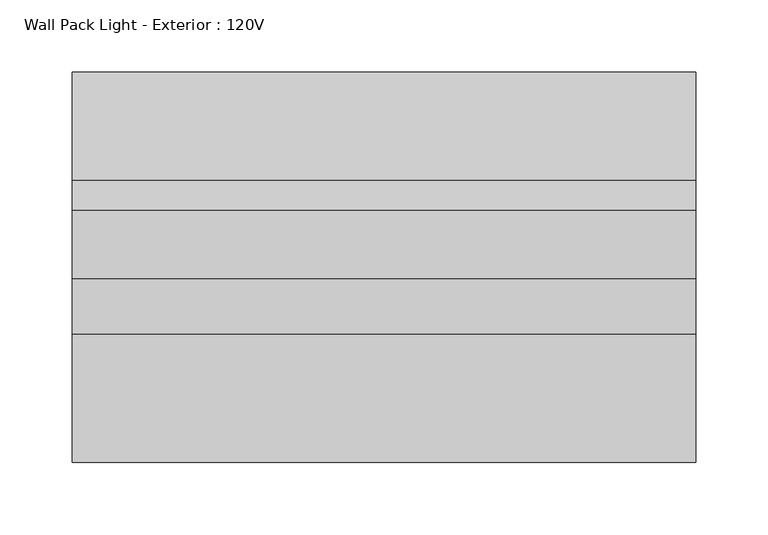
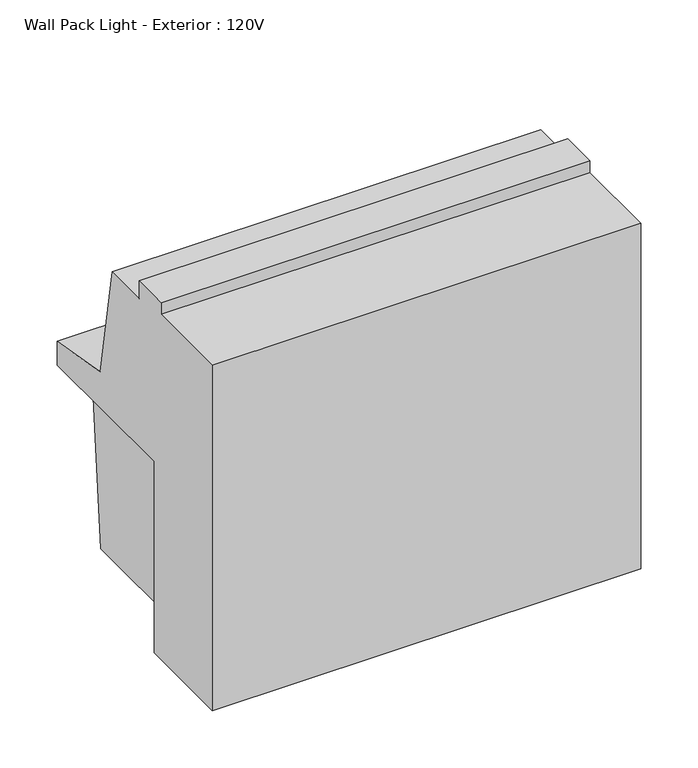
"""IFC4 building model written with IfcOpenShell, lengths in millimetres: light fixture geometry, Wall Pack Light - Exterior : 120V."""

from ifc_helpers import new_model, si_unit, frame, origin, place, context, project, spatial, polyline, outline, extrude, source, transform, mapped, element, save


def wall_pack_light_exterior_120v_50d39a1a(model_context):
    return source(origin(), model_context, "Body", "SweptSolid", [
        extrude(outline(polyline([(340.420745, 2393.95), (203.2, 2393.95), (203.2, 2578.1), (355.5170754, 2578.1), (340.420745, 2393.95)])), frame((-68.7349223, 0.0, 0.0), z_axis=(1.0, 0.0, 0.0), x_axis=(0.0, 1.0, 0.0)), (0.0, 0.0, 1.0), 380.9989788),
        extrude(outline(polyline([(190.5, 2755.9), (228.6, 2755.9), (228.6, 2736.85), (276.040971, 2736.85), (297.0426549, 2617.7435323), (372.0850056, 2604.5115412), (372.0850056, 2579.1115412), (203.2, 2579.1115412), (203.2, 2374.9), (101.6, 2374.9), (101.6, 2743.2), (190.5, 2743.2), (190.5, 2755.9)])), frame((-94.1359435, 0.0, 0.0), z_axis=(1.0, 0.0, 0.0), x_axis=(0.0, 1.0, 0.0)), (0.0, 0.0, 1.0), 431.8),
    ])


if __name__ == "__main__":
    model = new_model("IFC4")
    model_context = context("Model", 3, world=origin())
    ifc_project = project(units=[si_unit("LENGTHUNIT", "METRE", prefix="MILLI")], contexts=[model_context])
    site = spatial("IfcSite", under=ifc_project)
    building = spatial("IfcBuilding", under=site)
    placement = place(None, origin())
    wall_pack_light_exterior_120v_shape = wall_pack_light_exterior_120v_50d39a1a(model_context)
    element("IfcLightFixture", 1, ObjectType="Wall Pack Light - Exterior : 120V", at=placement, inside=building, context=model_context, shape_type="MappedRepresentation", body=[
        mapped(wall_pack_light_exterior_120v_shape, transform((0.0, 0.0, 0.0), x_axis=(1.0, 0.0, 0.0), y_axis=(0.0, 1.0, 0.0), z_axis=(0.0, 0.0, 1.0))),
    ])
    save(model, "model.ifc")

# Revit data of these elements
# Type "Wall Pack Light - Exterior : 120V"
#   Assembly Code = "D5020230"
#   Wattage = 70 W
#   built-in parameter 1150110 = 1 (stored number, unit not read)
#   built-in parameter 1114217 = 1 (stored number, unit not read)
#   built-in parameter 1150109 = 1 (stored number, unit not read)
#   built-in parameter 1150113 = 1 (stored number, unit not read)
#   built-in parameter 1150115 = 1 (stored number, unit not read)
#   built-in parameter 1150105 = 437.668 (stored number, unit not read)
#   Light Source Symbol Size = 2' - 0"
#   built-in parameter 1150112 = 1 (stored number, unit not read)
#   built-in parameter 1150114 = 1 (stored number, unit not read)
#   built-in parameter 1150107 = 4000 (stored number, unit not read)
#   built-in parameter 1150106 = 4.37668 (stored number, unit not read)
#   built-in parameter 1150104 = 7.29939 (stored number, unit not read)
#   Ballast Voltage = 120 V
#   built-in parameter 1114218 = 1 (stored number, unit not read)
#   built-in parameter 1150133 = 10 (stored number, unit not read)
#   Lumens = 5499.9 lm
#   Mounting Height = 9' - 0"
#   Apparent Load = 70 VA
#   built-in parameter 1150134 = 12
#   built-in parameter 1150137 = 1
#   Color Filter = 16777215
#   Ballast Number of Poles = 1
#   Wall Mount Material = Metal - Paint Finish - Dark Grey, Matte
#   Shade Material = Glass
#   Load Classification = Lighting - Exterior
#   Dimming Lamp Color Temperature Shift = (empty or 0)
#   Default Elevation = 0
# Element 1 (IfcLightFixture, "Wall Pack Light - Exterior : 120V")
#   Materials on its faces: "Metal - Paint Finish - Dark Grey, Matte", "Glass"
# Materials
#   "Metal - Paint Finish - Dark Grey, Matte": class "Paint", colour RGB 98 98 98, transparency 0
#   "Glass": class "Glass", colour RGB 0 128 192, transparency 0.75, Description = "Soda Lime Glass", Cost = 0
